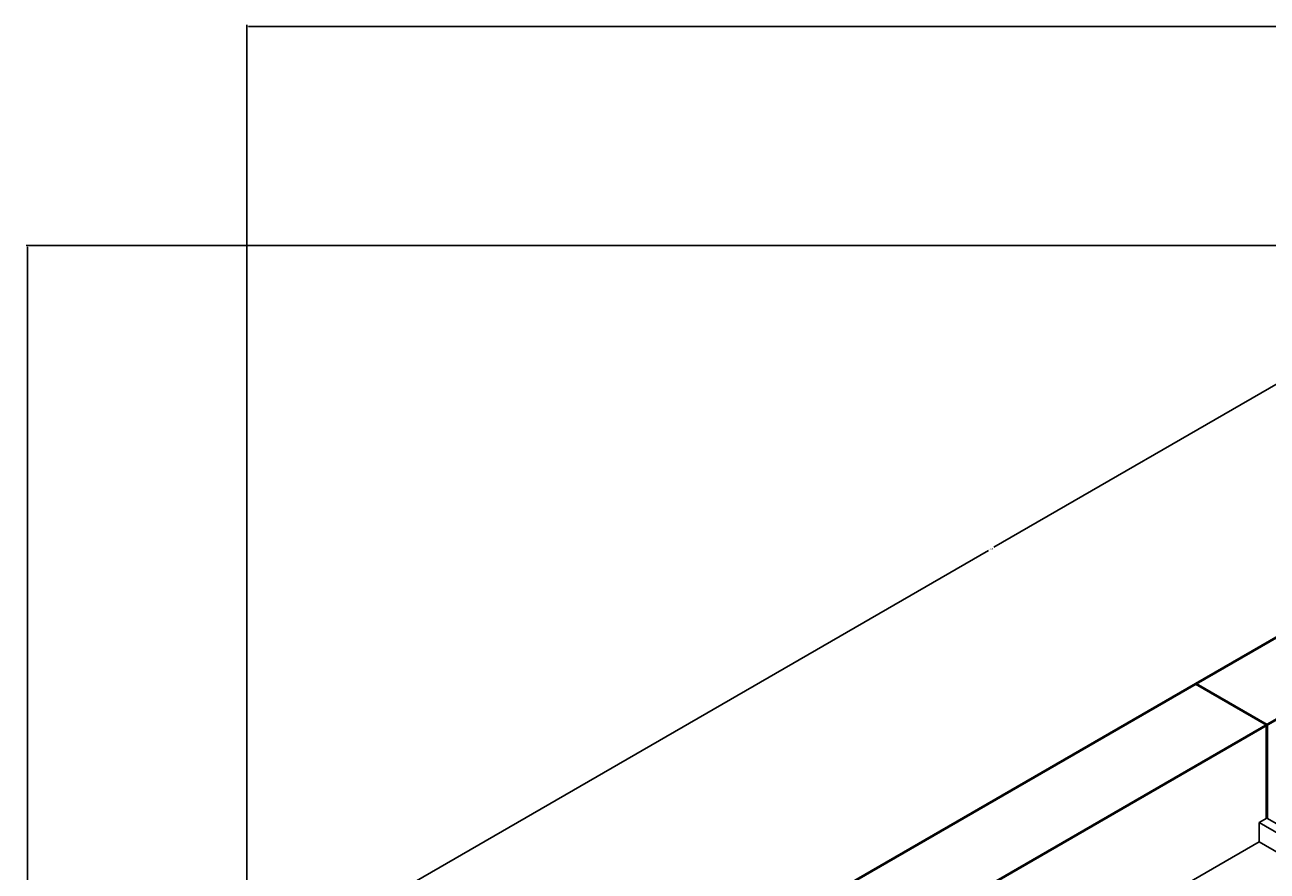
# Model space of a CAD drawing. Units: inches. Extents: x 4150 to 4636, y 2169 to 2592.
# Tile 4 of 8: x 4150 to 4286, y 2499 to 2592. Entities that reach past the tile are written whole.
import ezdxf

# ---------------------------------------------------------------- set-up
doc = ezdxf.new("R2010")
doc.units = ezdxf.units.IN
for name, color, linetype, lineweight in [('A-ANNO-DIMS', 2, 'Continuous', 18), ('A-FLOR-CASE', 3, 'Continuous', 25), ('A-WALL', 7, 'Continuous', 50)]:
    doc.layers.add(name, color=color, linetype=linetype, lineweight=lineweight)
doc.styles.get("Standard").update_dxf_attribs({"font": 'arial.ttf'})
doc.dimstyles.get("Standard").update_dxf_attribs({"dimtxt": 0.18, "dimasz": 0.18, "dimexe": 0.18, "dimexo": 0.0625, "dimgap": 0.09, "dimtad": 0, "dimtih": 1, "dimtoh": 1, "dimdec": 4, "dimzin": 0, "dimdsep": 46, "dimtxsty": 'Standard', "dimcen": 0.09, "dimadec": 0, "dimazin": 0, "dimtfac": 1, "dimtdec": 4, "dimtofl": 0, "dimtmove": 0, "dimatfit": 3, "dimfxl": 1, "dimtolj": 1, "dimtzin": 0, "dimarcsym": 0})

# ---------------------------------------------------------------- blocks, each defined once
blk = doc.blocks.new('CUBOARD 1')
for p, q in [((4285.13, 2504.76), (4286, 2505.26)), ((4285.13, 2502.65), (4285.13, 2504.76)), ((4293.79, 2499.76), (4285.13, 2504.76)), ((4295.52, 2499.76), (4286, 2505.26)), ((4262.66, 2489.68), (4285.13, 2502.65)), ((4291.96, 2498.71), (4285.13, 2502.65)), ((4269.49, 2485.74), (4293.79, 2499.76)), ((4270.36, 2485.24), (4295.52, 2499.76)), ((4270.36, 2485.24), (4295.52, 2499.76)), ((4295.52, 2499.76), (4295.52, 2496.65)), ((4270.36, 2482.12), (4295.52, 2496.65)), ((4294.66, 2496.15), (4294.66, 2461.49)), ((4284.67, 2488.39), (4292.93, 2493.15)), ((4292.93, 2493.15), (4292.93, 2462.49)), ((4259.97, 2491.24), (4270.36, 2485.24)), ((4259.97, 2488.12), (4259.97, 2491.24)), ((4282.94, 2489.39), (4282.94, 2454.72)), ((4284.67, 2488.39), (4284.67, 2457.72)), ((4259.97, 2488.12), (4270.36, 2482.12)), ((4259.97, 2488.12), (4259.97, 2459.23)), ((4272.96, 2481.62), (4281.21, 2486.39)), ((4281.21, 2486.39), (4281.21, 2455.72)), ((4270.36, 2485.24), (4270.36, 2482.12)), ((4270.36, 2482.12), (4270.36, 2485.24)), ((4270.36, 2482.12), (4270.36, 2453.23)), ((4271.22, 2482.62), (4271.22, 2452.73)), ((4272.96, 2481.62), (4272.96, 2451.73)), ((4275.13, 2450.21), (4294.66, 2461.49)), ((4284.67, 2457.72), (4292.93, 2462.49)), ((4273.63, 2451.35), (4281.21, 2455.72))]:
    blk.add_line(p, q)
for centre, radius, start, end in [((4281.84, 2459.9), 0.201, 29.3135, 156.7087), ((4283.56, 2460.89), 0.201, 29.3135, 156.7087), ((4283.63, 2457.8), 0.198, 207.8897, 338.1325), ((4281.92, 2456.81), 0.198, 207.8897, 338.1325)]:
    blk.add_arc(centre, radius, start, end)
for points in [[(4281.66, 2459.98), (4281.81, 2459.8), (4282.19, 2459.37), (4282.21, 2458.32), (4282.21, 2457.34), (4281.84, 2456.84), (4281.74, 2456.71)], [(4282.02, 2460), (4282.17, 2459.82), (4282.55, 2459.39), (4282.57, 2458.34), (4282.57, 2457.35), (4282.2, 2456.86), (4282.1, 2456.73)], [(4283.37, 2460.97), (4283.53, 2460.79), (4283.91, 2460.36), (4283.93, 2459.31), (4283.92, 2458.33), (4283.56, 2457.83), (4283.46, 2457.7)], [(4283.73, 2460.99), (4283.89, 2460.81), (4284.27, 2460.38), (4284.29, 2459.33), (4284.28, 2458.34), (4283.91, 2457.85), (4283.82, 2457.72)]]:
    blk.add_open_spline(points, degree=3, knots=[0, 0, 0, 0, 0.695815, 1.679053, 3.025679, 3.502598, 3.502598, 3.502598, 3.502598])
blk = doc.blocks.new('*D36')
at = {"layer": 'A-ANNO-DIMS', "color": 0, "lineweight": -2, "transparency": 16777216}
for p, q in [((4174.28, 2460.03), (4174.28, 2592.15)), ((4174.46, 2591.97), (4402.51, 2591.97)), ((4631.36, 2591.97), (4403.31, 2591.97)), ((4631.54, 2412.03), (4631.54, 2592.15))]:
    blk.add_line(p, q, dxfattribs=at)
at = {"layer": 'A-ANNO-DIMS', "color": 0, "transparency": 16777216}
for points in [[(4174.46, 2592), (4174.46, 2591.94), (4174.28, 2591.97)], [(4631.36, 2592), (4631.36, 2591.94), (4631.54, 2591.97)]]:
    blk.add_solid(points, dxfattribs=at)
at = {"layer": 'Defpoints', "color": 0, "transparency": 16777216}
for p in [(4631.54, 2591.97), (4174.28, 2459.97), (4631.54, 2411.97)]:
    blk.add_point(p, dxfattribs=at)
at = {"layer": 'A-ANNO-DIMS', "color": 0, "transparency": 16777216, "insert": (4402.91, 2591.97), "char_height": 0.18, "attachment_point": 5}
blk.add_mtext('\\A1;457.3', dxfattribs=at)
blk = doc.blocks.new('*D37')
at = {"layer": 'A-ANNO-DIMS', "color": 0, "lineweight": -2, "transparency": 16777216}
for p, q in [((4361.28, 2567.97), (4150.1, 2567.97)), ((4150.28, 2567.79), (4150.28, 2379.06)), ((4150.28, 2189.96), (4150.28, 2378.69)), ((4434.34, 2189.78), (4150.1, 2189.78))]:
    blk.add_line(p, q, dxfattribs=at)
at = {"layer": 'A-ANNO-DIMS', "color": 0, "transparency": 16777216}
for points in [[(4150.25, 2567.79), (4150.31, 2567.79), (4150.28, 2567.97)], [(4150.25, 2189.96), (4150.31, 2189.96), (4150.28, 2189.78)]]:
    blk.add_solid(points, dxfattribs=at)
at = {"layer": 'Defpoints', "color": 0, "transparency": 16777216}
for p in [(4361.34, 2567.97), (4150.28, 2189.78), (4434.4, 2189.78)]:
    blk.add_point(p, dxfattribs=at)
at = {"layer": 'A-ANNO-DIMS', "color": 0, "transparency": 16777216, "insert": (4150.28, 2378.87), "char_height": 0.18, "attachment_point": 5}
blk.add_mtext('\\A1;378.2', dxfattribs=at)
blk = doc.blocks.new('*D42')
at = {"layer": 'A-ANNO-DIMS', "color": 0, "lineweight": -2, "transparency": 16777216}
for p, q in [((4349.19, 2588.66), (4256.1, 2534.92)), ((4361.31, 2568.02), (4349.25, 2588.91)), ((4162.44, 2480.84), (4255.52, 2534.58)), ((4174.25, 2460.02), (4162.19, 2480.91))]:
    blk.add_line(p, q, dxfattribs=at)
at = {"layer": 'A-ANNO-DIMS', "color": 0, "transparency": 16777216}
for points in [[(4349.17, 2588.69), (4349.2, 2588.63), (4349.34, 2588.75)], [(4162.42, 2480.87), (4162.45, 2480.81), (4162.28, 2480.75)]]:
    blk.add_solid(points, dxfattribs=at)
at = {"layer": 'Defpoints', "color": 0, "transparency": 16777216}
for p in [(4349.34, 2588.75), (4361.34, 2567.97), (4174.28, 2459.97)]:
    blk.add_point(p, dxfattribs=at)
at = {"layer": 'A-ANNO-DIMS', "color": 0, "transparency": 16777216, "insert": (4255.81, 2534.75), "char_height": 0.18, "attachment_point": 5}
blk.add_mtext('\\A1;216', dxfattribs=at)

msp = doc.modelspace()

# ---------------------------------------------------------------- linework, layer by layer
at = {"layer": 'A-WALL'}
for p, q in [((4278.203, 2519.9652), (4361.3415, 2567.9652)), ((4182.0742, 2455.4652), (4361.3415, 2558.9652)), ((4174.28, 2459.9652), (4278.203, 2519.9652)), ((4278.203, 2519.9652), (4285.9973, 2515.4652)), ((4285.9973, 2515.4652), (4285.9973, 2505.2646))]:
    msp.add_line(p, q, dxfattribs=at)

# ---------------------------------------------------------------- block references
at = {"layer": 'A-FLOR-CASE'}
msp.add_blockref('CUBOARD 1', (0, 0), dxfattribs=at)

# ---------------------------------------------------------------- dimensions: what is measured, and where the dimension line sits
at = {"layer": 'A-ANNO-DIMS'}
dim = msp.add_linear_dim(base=(4631.5414, 2591.9652), p1=(4174.28, 2459.9652), p2=(4631.5414, 2411.9652), dimstyle='Standard', override={"dimdec": 1, "dimlfac": 1, "dimrnd": 0, "dimzin": 0, "dimdsep": 46, "dimlunit": 2}, dxfattribs=at)
dim.commit()
dim.dimension.update_dxf_attribs({"geometry": '*D36', "text_midpoint": (4402.9107, 2591.9652)})
for base, p1, p2, angle, override, picture, middle in [((4349.3415, 2588.7498), (4174.28, 2459.9652), (4361.3415, 2567.9652), 30, {"dimdec": 0, "dimlfac": 1, "dimrnd": 0, "dimzin": 0, "dimdsep": 46, "dimlunit": 2}, '*D42', (4255.8107, 2534.7498)), ((4150.28, 2189.7836), (4361.3415, 2567.9652), (4434.4021, 2189.7836), 90, {"dimdec": 1, "dimlfac": 1, "dimrnd": 0, "dimzin": 0, "dimdsep": 46, "dimlunit": 2}, '*D37', (4150.28, 2378.8744))]:
    dim = msp.add_linear_dim(base=base, p1=p1, p2=p2, angle=angle, dimstyle='Standard', override=override, dxfattribs=at)
    dim.commit()
    dim.dimension.update_dxf_attribs({"geometry": picture, "text_midpoint": middle})

doc.saveas('drawing.dxf')
